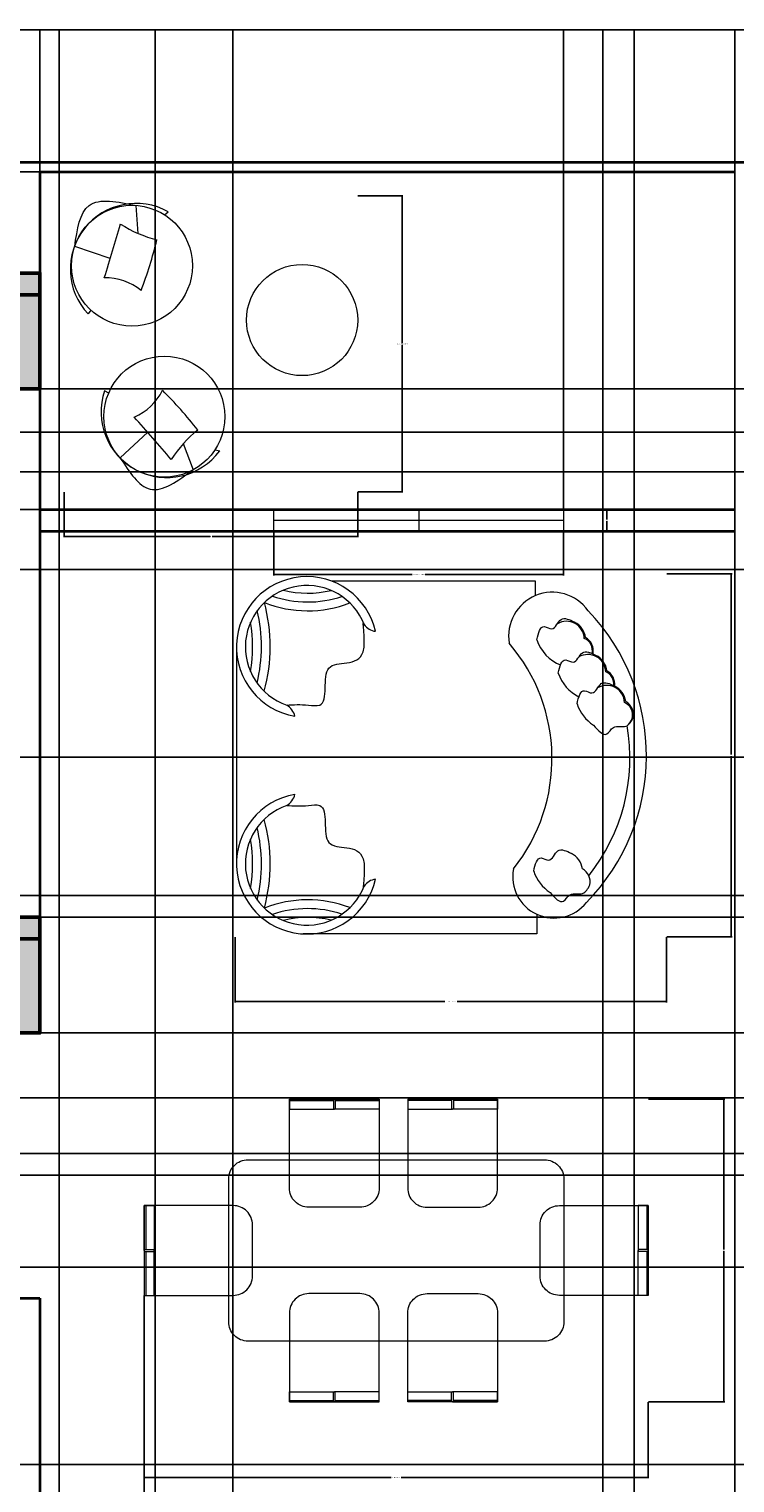
# Model space of a CAD drawing. Units: inches. Extents: x 393 to 993, y 153 to 660.
# Tile 4 of 6: x 645 to 791, y 359 to 660. Entities that reach past the tile are written whole.
import ezdxf

# ---------------------------------------------------------------- set-up
doc = ezdxf.new("R2010")
doc.units = ezdxf.units.IN
doc.header["$MEASUREMENT"] = 0
for name, color, linetype, lineweight in [('A-ANNO-DIMS', 2, 'Continuous', 18), ('A-COLS', 40, 'Continuous', 50), ('A-GLAZ', 4, 'Continuous', 20), ('A-WALL', 40, 'Continuous', 35), ('FURNITURE', 72, 'Continuous', 18)]:
    doc.layers.add(name, color=color, linetype=linetype, lineweight=lineweight)
doc.styles.get("Standard").update_dxf_attribs({"font": 'arial.ttf'})
doc.dimstyles.get("Standard").update_dxf_attribs({"dimtxt": 0.18, "dimasz": 0.18, "dimexe": 0.18, "dimexo": 0.0625, "dimgap": 0.09, "dimtad": 0, "dimtih": 1, "dimtoh": 1, "dimdec": 1, "dimzin": 0, "dimdsep": 46, "dimlunit": 3, "dimtxsty": 'Standard', "dimcen": 0.09, "dimadec": 0, "dimazin": 0, "dimtfac": 1, "dimtdec": 1, "dimtofl": 0, "dimtmove": 0, "dimatfit": 3, "dimfxl": 1, "dimtolj": 1, "dimtzin": 0, "dimarcsym": 0})

# ---------------------------------------------------------------- blocks, each defined once
blk = doc.blocks.new('YY')
for p, q in [((725.97, 560.91), (725.97, 558.66)), ((695.97, 558.66), (725.97, 558.66)), ((725.97, 558.66), (725.97, 556.41)), ((725.97, 558.66), (755.97, 558.66))]:
    blk.add_line(p, q)
blk.add_lwpolyline([(695.97, 556.41), (695.97, 560.91), (755.97, 560.91), (755.97, 556.41), (695.97, 556.41)])
blk = doc.blocks.new('SS')
for p, q in [((702.19, 481.41), (711.3, 481.41)), ((711.3, 481.71), (711.3, 479.62)), ((711.7, 481.71), (711.7, 479.62)), ((711.7, 481.41), (720.8, 481.41)), ((735.8, 481.41), (726.7, 481.41)), ((735.8, 481.71), (735.8, 479.62)), ((736.2, 481.71), (736.2, 479.62)), ((745.31, 481.41), (736.2, 481.41)), ((672.41, 459.62), (672.41, 450.52)), ((776.25, 459.62), (776.25, 450.52)), ((672.11, 450.52), (674.19, 450.52)), ((672.11, 450.12), (674.19, 450.12)), ((672.41, 450.12), (672.41, 441.01)), ((776.55, 450.52), (774.47, 450.52)), ((776.55, 450.12), (774.47, 450.12)), ((776.25, 450.12), (776.25, 441.01)), ((702.19, 419.23), (711.3, 419.23)), ((711.3, 418.93), (711.3, 421.02)), ((711.7, 418.93), (711.7, 421.02)), ((711.7, 419.23), (720.8, 419.23)), ((735.8, 419.23), (726.7, 419.23)), ((735.8, 418.93), (735.8, 421.02)), ((736.2, 418.93), (736.2, 421.02)), ((745.31, 419.23), (736.2, 419.23))]:
    blk.add_line(p, q)
for points in [[(702.19, 481.71), (720.8, 481.71), (720.8, 463.27, -0.414214), (716.8, 459.27), (706.19, 459.27, -0.414214), (702.19, 463.27)], [(745.31, 481.71), (726.7, 481.71), (726.7, 463.27, 0.414214), (730.7, 459.27), (741.31, 459.27, 0.414214), (745.31, 463.27)], [(693.61, 469.12), (755.05, 469.12, -0.414214), (759.05, 465.12), (759.05, 435.52, -0.414214), (755.05, 431.52), (693.61, 431.52, -0.414214), (689.61, 435.52), (689.61, 465.12, -0.414214)], [(672.11, 459.62), (672.11, 441.01), (690.54, 441.01, 0.414214), (694.54, 445.01), (694.54, 455.62, 0.414214), (690.54, 459.62)], [(776.55, 459.62), (776.55, 441.01), (758.12, 441.01, -0.414214), (754.12, 445.01), (754.12, 455.62, -0.414214), (758.12, 459.62)], [(702.19, 418.93), (720.8, 418.93), (720.8, 437.36, 0.414214), (716.8, 441.36), (706.19, 441.36, 0.414214), (702.19, 437.36)], [(745.31, 418.93), (726.7, 418.93), (726.7, 437.36, -0.414214), (730.7, 441.36), (741.31, 441.36, -0.414214), (745.31, 437.36)]]:
    blk.add_lwpolyline(points, format="xyb", close=True)
for points in [[(711.5, 481.71), (702.19, 481.71), (702.19, 479.62), (711.5, 479.62)], [(711.5, 481.71), (720.8, 481.71), (720.8, 479.62), (711.5, 479.62)], [(736, 481.71), (726.7, 481.71), (726.7, 479.62), (736, 479.62)], [(736, 481.71), (745.31, 481.71), (745.31, 479.62), (736, 479.62)], [(672.11, 450.32), (672.11, 459.62), (674.19, 459.62), (674.19, 450.32)], [(776.55, 450.32), (776.55, 459.62), (774.47, 459.62), (774.47, 450.32)], [(672.11, 450.32), (672.11, 441.01), (674.19, 441.01), (674.19, 450.32)], [(776.55, 450.32), (776.55, 441.01), (774.47, 441.01), (774.47, 450.32)], [(711.5, 418.93), (702.19, 418.93), (702.19, 421.02), (711.5, 421.02)], [(711.5, 418.93), (720.8, 418.93), (720.8, 421.02), (711.5, 421.02)], [(736, 418.93), (726.7, 418.93), (726.7, 421.02), (736, 421.02)], [(736, 418.93), (745.31, 418.93), (745.31, 421.02), (736, 421.02)]]:
    blk.add_lwpolyline(points)
blk = doc.blocks.new('CC')
for p, q in [((667.82, 618.13), (667.42, 623.92)), ((673.29, 621.98), (674.07, 622.6)), ((662.05, 612.95), (654.68, 615.45)), ((658.03, 602.24), (657.45, 601.43)), ((661.73, 585.02), (660.87, 585.52)), ((669.8, 576.91), (664.12, 571.6)), ((677.19, 574.56), (679.21, 569.12)), ((683.76, 573.3), (684.73, 573.06))]:
    blk.add_line(p, q)
for centre, radius in [((666.54, 611.43), 12.53), ((701.8, 600.17), 11.52), ((673.27, 580.15), 12.53)]:
    blk.add_circle(centre, radius)
for centre, radius, start, end in [((667.39, 610.73), 13.62, 60.6306, 223.0738), ((-908.47, 1091.34), 1641.76, 342.91261, 343.31902), ((677.83, 641.08), 25.04, 237.0171, 255.8371), ((587.69, 637.23), 86.46, 339.0342, 346.3342), ((660.99, 597.14), 11.8, 50.9057, 90.8219), ((673.76, 581.14), 13.62, 161.2133, 323.6564), ((662.33, 590.89), 11.8, 293.4651, 333.3813), ((612.01, 524.2), 86.46, 37.9528, 45.2528), ((-564.96, -505.1), 1641.76, 40.968, 41.3744), ((695.76, 557.76), 25.04, 128.4499, 147.2699)]:
    blk.add_arc(centre, radius, start, end)
for points in [[(654.68, 615.45), (655.2, 618.95), (656.28, 626.24), (663.61, 624.72), (667.42, 623.92)], [(664.12, 571.6), (666.03, 568.63), (670.01, 562.43), (676.06, 566.83), (679.21, 569.12)]]:
    blk.add_open_spline(points, degree=3, knots=[0, 0, 0, 0, 8.969281, 18.721099, 18.721099, 18.721099, 18.721099])
blk = doc.blocks.new('ll')
at = {"layer": 'FURNITURE'}
for p, q in [((750.18, 546.06), (707.9, 546.06)), ((750.18, 543.06), (750.18, 546.06)), ((688.21, 532.4), (688.21, 487.49)), ((750.42, 477.01), (750.42, 472.96)), ((750.42, 472.96), (702.01, 472.96))]:
    blk.add_line(p, q, dxfattribs=at)
for centre, radius, start, end in [((702.79, 532.4), 14.58, 12.8767, 260.2291), ((702.79, 532.4), 12.75, 21.3555, 250.8998), ((702.95, 564.16), 22.43, 250.9613, 288.4654), ((702.95, 564.16), 20.6, 255.8439, 283.5828), ((753.65, 534.69), 9.06, 35.3162, 189.6304), ((660.81, 532.52), 32.56, 346.4953, 13.1907), ((660.81, 532.52), 34.39, 344.3453, 15.3407), ((702.95, 564.16), 24.26, 248.2968, 291.1299), ((729.74, 509.85), 43.41, 315.5068, 43.8598), ((660.81, 532.52), 30.73, 350.2595, 9.4265), ((717.38, 538.95), 3.32, 214.9691, 263.4589), ((756.58, 534.03), 3.7, 2.2519, 120.5397), ((756.43, 533.85), 4.13, 7.2046, 63.8494), ((758.42, 536.54), 8.42, 198.3753, 248.7655), ((759.17, 531.63), 2.78, 348.3194, 66.5647), ((758.97, 531.6), 3.17, 349.5851, 60.6705), ((716.9, 509.26), 36.68, 321.4717, 40.6866), ((761.02, 527.14), 3.7, 2.2519, 120.5397), ((760.86, 526.95), 4.13, 7.2046, 63.8494), ((763.41, 524.7), 3.17, 352.5529, 60.6705), ((762.86, 529.64), 8.42, 198.3753, 243.944), ((764.92, 520.75), 3.7, 2.2519, 120.5397), ((763.61, 524.73), 2.78, 352.8755, 66.5647), ((763.61, 524.73), 2.78, 348.3194, 348.3993), ((764.76, 520.57), 4.13, 7.2046, 63.8494), ((696.54, 517.06), 3.9, 14.5272, 57.8422), ((766.76, 523.26), 8.42, 198.3753, 236.9846), ((767.51, 518.34), 2.78, 305.7015, 66.5647), ((767.31, 518.32), 3.17, 349.5851, 60.6705), ((730.58, 509.37), 39.14, 321.4898, 9.8869), ((702.79, 487.49), 14.58, 99.7709, 347.1233), ((696.54, 502.84), 3.9, 302.1578, 345.4728), ((702.79, 487.49), 12.75, 109.1002, 338.6445), ((660.81, 487.38), 32.56, 346.8093, 13.5047), ((660.81, 487.38), 34.39, 344.6593, 15.6547), ((660.81, 487.38), 30.73, 350.5735, 9.7405), ((755.78, 485.9), 4.13, 7.2046, 63.8494), ((754.02, 484.79), 8.58, 169.1466, 321.2907), ((757.78, 488.59), 8.42, 198.3753, 236.9846), ((758.33, 483.65), 3.17, 349.5851, 60.6705), ((717.38, 480.95), 3.32, 96.5411, 145.0309), ((702.95, 455.74), 24.26, 68.8701, 111.7032), ((702.95, 455.74), 22.43, 71.5346, 109.0387), ((702.95, 455.74), 20.6, 76.4172, 104.1561)]:
    blk.add_arc(centre, radius, start, end, dxfattribs=at)
for points, knots in [([(698.62, 520.36), (700.04, 520.44), (702.22, 520.56), (707.91, 519.62), (704.27, 531.4), (716.71, 526.93), (714.02, 538.83), (714.69, 536.96), (714.71, 536.92)], [0, 0, 0, 0, 4.487467, 6.830013, 14.741049, 22.564713, 28.22617, 28.364822, 28.364822, 28.364822, 28.364822]), ([(750.43, 533.89), (750.76, 535.31), (751.27, 537.45), (754.08, 535.39), (755.19, 539.08), (757.21, 538.07), (758.25, 537.56)], [0, 0, 0, 0, 3.161517, 4.748893, 7.471418, 10.321278, 10.321278, 10.321278, 10.321278]), ([(754.86, 526.99), (755.2, 528.41), (755.71, 530.55), (758.51, 528.49), (759.63, 532.18), (761.65, 531.17), (762.68, 530.66)], [0, 0, 0, 0, 3.161517, 4.748893, 7.471418, 10.321278, 10.321278, 10.321278, 10.321278]), ([(758.77, 520.6), (759.1, 522.03), (759.61, 524.16), (762.42, 522.1), (763.53, 525.79), (765.55, 524.79), (766.59, 524.28)], [0, 0, 0, 0, 3.161517, 4.748893, 7.471418, 10.321278, 10.321278, 10.321278, 10.321278]), ([(762.17, 516.19), (763.19, 515.06), (764.77, 513.29), (766.27, 516.46), (769.11, 515.35), (770.01, 516.98), (770.43, 517.75)], [0, 0, 0, 0, 3.335346, 5.221215, 7.830033, 10.164656, 10.164656, 10.164656, 10.164656]), ([(698.62, 499.54), (700.04, 499.46), (702.22, 499.34), (707.91, 500.28), (704.27, 488.5), (716.71, 492.97), (714.02, 481.06), (714.69, 482.94), (714.71, 482.98)], [0, 0, 0, 0, 4.487467, 6.830013, 14.741049, 22.564713, 28.22617, 28.364822, 28.364822, 28.364822, 28.364822]), ([(749.79, 485.93), (750.12, 487.36), (750.63, 489.49), (753.43, 487.43), (754.55, 491.12), (756.57, 490.12), (757.61, 489.61)], [0, 0, 0, 0, 3.161517, 4.748893, 7.471418, 10.321278, 10.321278, 10.321278, 10.321278]), ([(753.19, 481.52), (754.21, 480.39), (755.79, 478.62), (757.28, 481.79), (760.13, 480.68), (761.03, 482.31), (761.45, 483.08)], [0, 0, 0, 0, 3.335346, 5.221215, 7.830033, 10.164656, 10.164656, 10.164656, 10.164656])]:
    blk.add_open_spline(points, degree=3, knots=knots, dxfattribs=at)
blk = doc.blocks.new('COL-9X24-RH')
h = blk.add_hatch(color=256)
h.dxf.hatch_style = 1
h.paths.add_polyline_path([(4.5, 19.5), (4.5, 24), (0, 24), (0, 0), (9, 0), (9, 19.5)])
h = blk.add_hatch(color=256)
h.dxf.hatch_style = 1
h.paths.add_polyline_path([(4.5, 19.5), (9, 19.5), (9, 24), (4.5, 24)])
for p, q in [((4.5, 24), (4.5, 19.5)), ((4.5, 24), (9, 24)), ((9, 24), (9, 19.5)), ((4.5, 19.5), (9, 19.5))]:
    blk.add_line(p, q)
blk.add_lwpolyline([(0, 24), (9, 24), (9, 0), (0, 0), (0, 24)])
blk = doc.blocks.new('*D28')
at = {"layer": 'A-ANNO-DIMS', "color": 0, "lineweight": -2, "transparency": 16777216}
for p, q in [((695.97, 556.34), (695.97, 547.23)), ((755.97, 556.34), (755.97, 547.23)), ((696.15, 547.41), (724.63, 547.41)), ((755.79, 547.41), (727.31, 547.41))]:
    blk.add_line(p, q, dxfattribs=at)
at = {"layer": 'A-ANNO-DIMS', "color": 0, "transparency": 16777216}
for points in [[(696.15, 547.44), (696.15, 547.38), (695.97, 547.41)], [(755.79, 547.44), (755.79, 547.38), (755.97, 547.41)]]:
    blk.add_solid(points, dxfattribs=at)
at = {"layer": 'Defpoints', "color": 0, "transparency": 16777216}
for p in [(695.97, 556.41), (755.97, 556.41), (755.97, 547.41)]:
    blk.add_point(p, dxfattribs=at)
at = {"layer": 'A-ANNO-DIMS', "color": 0, "transparency": 16777216, "insert": (725.97, 547.41), "char_height": 0.18, "attachment_point": 5}
blk.add_mtext('\\A1;BALCONY SLIDER 60', dxfattribs=at)
blk = doc.blocks.new('*D29')
at = {"layer": 'A-ANNO-DIMS', "color": 0, "lineweight": -2, "transparency": 16777216}
for p, q in [((756.03, 560.91), (765.15, 560.91)), ((764.97, 560.73), (764.97, 558.84)), ((764.97, 556.59), (764.97, 558.48)), ((756.03, 556.41), (765.15, 556.41))]:
    blk.add_line(p, q, dxfattribs=at)
at = {"layer": 'A-ANNO-DIMS', "color": 0, "transparency": 16777216}
for points in [[(764.94, 560.73), (765, 560.73), (764.97, 560.91)], [(764.94, 556.59), (765, 556.59), (764.97, 556.41)]]:
    blk.add_solid(points, dxfattribs=at)
at = {"layer": 'Defpoints', "color": 0, "transparency": 16777216}
for p in [(755.97, 560.91), (764.97, 560.91), (755.97, 556.41)]:
    blk.add_point(p, dxfattribs=at)
at = {"layer": 'A-ANNO-DIMS', "color": 0, "transparency": 16777216, "insert": (764.97, 558.66), "char_height": 0.18, "attachment_point": 5}
blk.add_mtext('\\A1;5', dxfattribs=at)
blk = doc.blocks.new('*D36')
at = {"layer": 'A-ANNO-DIMS', "color": 0, "lineweight": -2, "transparency": 16777216}
for p, q in [((669.09, 375.86), (669.09, 360.08)), ((773.53, 375.86), (773.53, 360.08)), ((669.27, 360.26), (720.27, 360.26)), ((773.35, 360.26), (722.35, 360.26))]:
    blk.add_line(p, q, dxfattribs=at)
at = {"layer": 'A-ANNO-DIMS', "color": 0, "transparency": 16777216}
for points in [[(669.27, 360.29), (669.27, 360.23), (669.09, 360.26)], [(773.35, 360.29), (773.35, 360.23), (773.53, 360.26)]]:
    blk.add_solid(points, dxfattribs=at)
at = {"layer": 'Defpoints', "color": 0, "transparency": 16777216}
for p in [(669.09, 375.92), (773.53, 375.92), (773.53, 360.26)]:
    blk.add_point(p, dxfattribs=at)
at = {"layer": 'A-ANNO-DIMS', "color": 0, "transparency": 16777216, "insert": (721.31, 360.26), "char_height": 0.18, "attachment_point": 5}
blk.add_mtext('\\A1;DINING SET 104', dxfattribs=at)
blk = doc.blocks.new('*D37')
at = {"layer": 'A-ANNO-DIMS', "color": 0, "lineweight": -2, "transparency": 16777216}
for p, q in [((773.6, 438.7), (789.38, 438.7)), ((789.2, 438.52), (789.2, 407.49)), ((789.2, 376.1), (789.2, 407.13)), ((773.6, 375.92), (789.38, 375.92))]:
    blk.add_line(p, q, dxfattribs=at)
at = {"layer": 'A-ANNO-DIMS', "color": 0, "transparency": 16777216}
for points in [[(789.17, 438.52), (789.23, 438.52), (789.2, 438.7)], [(789.17, 376.1), (789.23, 376.1), (789.2, 375.92)]]:
    blk.add_solid(points, dxfattribs=at)
at = {"layer": 'Defpoints', "color": 0, "transparency": 16777216}
for p in [(773.53, 438.7), (789.2, 438.7), (773.53, 375.92)]:
    blk.add_point(p, dxfattribs=at)
at = {"layer": 'A-ANNO-DIMS', "color": 0, "transparency": 16777216, "insert": (789.2, 407.31), "char_height": 0.18, "attachment_point": 5}
blk.add_mtext('\\A1;63', dxfattribs=at)
blk = doc.blocks.new('*D38')
at = {"layer": 'A-ANNO-DIMS', "color": 0, "lineweight": -2, "transparency": 16777216}
for p, q in [((713.38, 625.89), (722.7, 625.89)), ((722.52, 625.71), (722.52, 595.4)), ((722.52, 564.72), (722.52, 595.03)), ((713.38, 564.54), (722.7, 564.54))]:
    blk.add_line(p, q, dxfattribs=at)
at = {"layer": 'A-ANNO-DIMS', "color": 0, "transparency": 16777216}
for points in [[(722.49, 625.71), (722.55, 625.71), (722.52, 625.89)], [(722.49, 564.72), (722.55, 564.72), (722.52, 564.54)]]:
    blk.add_solid(points, dxfattribs=at)
at = {"layer": 'Defpoints', "color": 0, "transparency": 16777216}
for p in [(713.32, 625.89), (722.52, 625.89), (713.32, 564.54)]:
    blk.add_point(p, dxfattribs=at)
at = {"layer": 'A-ANNO-DIMS', "color": 0, "transparency": 16777216, "insert": (722.52, 595.22), "char_height": 0.18, "attachment_point": 5}
blk.add_mtext('\\A1;BALCONY SEATING 61', dxfattribs=at)
blk = doc.blocks.new('*D39')
at = {"layer": 'A-ANNO-DIMS', "color": 0, "lineweight": -2, "transparency": 16777216}
for p, q in [((652.53, 564.48), (652.53, 555.15)), ((713.32, 564.48), (713.32, 555.15)), ((652.71, 555.33), (682.72, 555.33)), ((713.14, 555.33), (683.13, 555.33))]:
    blk.add_line(p, q, dxfattribs=at)
at = {"layer": 'A-ANNO-DIMS', "color": 0, "transparency": 16777216}
for points in [[(652.71, 555.36), (652.71, 555.3), (652.53, 555.33)], [(713.14, 555.36), (713.14, 555.3), (713.32, 555.33)]]:
    blk.add_solid(points, dxfattribs=at)
at = {"layer": 'Defpoints', "color": 0, "transparency": 16777216}
for p in [(652.53, 564.54), (713.32, 564.54), (713.32, 555.33)]:
    blk.add_point(p, dxfattribs=at)
at = {"layer": 'A-ANNO-DIMS', "color": 0, "transparency": 16777216, "insert": (682.92, 555.33), "char_height": 0.18, "attachment_point": 5}
blk.add_mtext('\\A1;61', dxfattribs=at)
blk = doc.blocks.new('*D40')
at = {"layer": 'A-ANNO-DIMS', "color": 0, "lineweight": -2, "transparency": 16777216}
for p, q in [((687.93, 472.24), (687.93, 458.71)), ((777.32, 472.24), (777.32, 458.71)), ((688.11, 458.89), (731.35, 458.89)), ((777.14, 458.89), (733.9, 458.89))]:
    blk.add_line(p, q, dxfattribs=at)
at = {"layer": 'A-ANNO-DIMS', "color": 0, "transparency": 16777216}
for points in [[(688.11, 458.92), (688.11, 458.86), (687.93, 458.89)], [(777.14, 458.92), (777.14, 458.86), (777.32, 458.89)]]:
    blk.add_solid(points, dxfattribs=at)
at = {"layer": 'Defpoints', "color": 0, "transparency": 16777216}
for p in [(687.93, 472.3), (777.32, 472.3), (777.32, 458.89)]:
    blk.add_point(p, dxfattribs=at)
at = {"layer": 'A-ANNO-DIMS', "color": 0, "transparency": 16777216, "insert": (732.63, 458.89), "char_height": 0.18, "attachment_point": 5}
blk.add_mtext('\\A1;LOUNGE GROUP 89', dxfattribs=at)
blk = doc.blocks.new('*D41')
at = {"layer": 'A-ANNO-DIMS', "color": 0, "lineweight": -2, "transparency": 16777216}
for p, q in [((777.38, 547.6), (790.9, 547.6)), ((790.72, 547.42), (790.72, 510.13)), ((790.72, 472.48), (790.72, 509.77)), ((777.38, 472.3), (790.9, 472.3))]:
    blk.add_line(p, q, dxfattribs=at)
at = {"layer": 'A-ANNO-DIMS', "color": 0, "transparency": 16777216}
for points in [[(790.69, 547.42), (790.75, 547.42), (790.72, 547.6)], [(790.69, 472.48), (790.75, 472.48), (790.72, 472.3)]]:
    blk.add_solid(points, dxfattribs=at)
at = {"layer": 'Defpoints', "color": 0, "transparency": 16777216}
for p in [(777.32, 547.6), (790.72, 547.6), (777.32, 472.3)]:
    blk.add_point(p, dxfattribs=at)
at = {"layer": 'A-ANNO-DIMS', "color": 0, "transparency": 16777216, "insert": (790.72, 509.95), "char_height": 0.18, "attachment_point": 5}
blk.add_mtext('\\A1;75', dxfattribs=at)
blk = doc.blocks.new('*D48')
at = {"layer": 'A-ANNO-DIMS', "color": 0, "lineweight": -2, "transparency": 16777216}
for p, q in [((642.98, 632.97), (642.98, 660.49)), ((643.16, 660.31), (719.2, 660.31)), ((795.8, 660.31), (719.76, 660.31)), ((795.98, 632.97), (795.98, 660.49))]:
    blk.add_line(p, q, dxfattribs=at)
at = {"layer": 'A-ANNO-DIMS', "color": 0, "transparency": 16777216}
for points in [[(643.16, 660.34), (643.16, 660.28), (642.98, 660.31)], [(795.8, 660.34), (795.8, 660.28), (795.98, 660.31)]]:
    blk.add_solid(points, dxfattribs=at)
at = {"layer": 'Defpoints', "color": 0, "transparency": 16777216}
for p in [(795.98, 660.31), (642.98, 632.91), (795.98, 632.91)]:
    blk.add_point(p, dxfattribs=at)
at = {"layer": 'A-ANNO-DIMS', "color": 0, "transparency": 16777216, "insert": (719.48, 660.31), "char_height": 0.18, "attachment_point": 5}
blk.add_mtext('\\A1;153', dxfattribs=at)
blk = doc.blocks.new('*D55')
at = {"layer": 'A-ANNO-DIMS', "color": 0, "lineweight": -2, "transparency": 16777216}
for p, q in [((791.42, 630.91), (393.4, 630.91)), ((393.58, 630.73), (393.58, 596.09)), ((393.58, 561.09), (393.58, 595.72)), ((791.42, 560.91), (393.4, 560.91))]:
    blk.add_line(p, q, dxfattribs=at)
at = {"layer": 'A-ANNO-DIMS', "color": 0, "transparency": 16777216}
for points in [[(393.55, 630.73), (393.61, 630.73), (393.58, 630.91)], [(393.55, 561.09), (393.61, 561.09), (393.58, 560.91)]]:
    blk.add_solid(points, dxfattribs=at)
at = {"layer": 'Defpoints', "color": 0, "transparency": 16777216}
for p in [(791.48, 630.91), (393.58, 560.91), (791.48, 560.91)]:
    blk.add_point(p, dxfattribs=at)
at = {"layer": 'A-ANNO-DIMS', "color": 0, "transparency": 16777216, "insert": (393.58, 595.91), "char_height": 0.18, "attachment_point": 5}
blk.add_mtext('\\A1;70', dxfattribs=at)
blk = doc.blocks.new('*D59')
at = {"layer": 'A-ANNO-DIMS', "color": 0, "lineweight": -2, "transparency": 16777216}
for p, q in [((651.48, 185.47), (651.48, 660.49)), ((651.66, 660.31), (669.26, 660.31)), ((687.3, 660.31), (669.7, 660.31)), ((687.48, 185.47), (687.48, 660.49))]:
    blk.add_line(p, q, dxfattribs=at)
at = {"layer": 'A-ANNO-DIMS', "color": 0, "transparency": 16777216}
for points in [[(651.66, 660.34), (651.66, 660.28), (651.48, 660.31)], [(687.3, 660.34), (687.3, 660.28), (687.48, 660.31)]]:
    blk.add_solid(points, dxfattribs=at)
at = {"layer": 'Defpoints', "color": 0, "transparency": 16777216}
for p in [(687.48, 660.31), (651.48, 185.41), (687.48, 185.41)]:
    blk.add_point(p, dxfattribs=at)
at = {"layer": 'A-ANNO-DIMS', "color": 0, "transparency": 16777216, "insert": (669.48, 660.31), "char_height": 0.18, "attachment_point": 5}
blk.add_mtext('\\A1;36', dxfattribs=at)
blk = doc.blocks.new('*D62')
at = {"layer": 'A-ANNO-DIMS', "color": 0, "lineweight": -2, "transparency": 16777216}
for p, q in [((848.42, 422.91), (393.4, 422.91)), ((393.58, 422.73), (393.58, 393.09)), ((393.58, 363.09), (393.58, 392.72)), ((848.42, 362.91), (393.4, 362.91))]:
    blk.add_line(p, q, dxfattribs=at)
at = {"layer": 'A-ANNO-DIMS', "color": 0, "transparency": 16777216}
for points in [[(393.55, 422.73), (393.61, 422.73), (393.58, 422.91)], [(393.55, 363.09), (393.61, 363.09), (393.58, 362.91)]]:
    blk.add_solid(points, dxfattribs=at)
at = {"layer": 'Defpoints', "color": 0, "transparency": 16777216}
for p in [(393.58, 422.91), (848.48, 422.91), (848.48, 362.91)]:
    blk.add_point(p, dxfattribs=at)
at = {"layer": 'A-ANNO-DIMS', "color": 0, "transparency": 16777216, "insert": (393.58, 392.91), "char_height": 0.18, "attachment_point": 5}
blk.add_mtext('\\A1;60', dxfattribs=at)
blk = doc.blocks.new('*D63')
at = {"layer": 'A-ANNO-DIMS', "color": 0, "lineweight": -2, "transparency": 16777216}
for p, q in [((960.92, 476.41), (393.4, 476.41)), ((393.58, 476.23), (393.58, 452.09)), ((393.58, 427.59), (393.58, 451.72)), ((960.92, 427.41), (393.4, 427.41))]:
    blk.add_line(p, q, dxfattribs=at)
at = {"layer": 'A-ANNO-DIMS', "color": 0, "transparency": 16777216}
for points in [[(393.55, 476.23), (393.61, 476.23), (393.58, 476.41)], [(393.55, 427.59), (393.61, 427.59), (393.58, 427.41)]]:
    blk.add_solid(points, dxfattribs=at)
at = {"layer": 'Defpoints', "color": 0, "transparency": 16777216}
for p in [(393.58, 476.41), (960.98, 476.41), (960.98, 427.41)]:
    blk.add_point(p, dxfattribs=at)
at = {"layer": 'A-ANNO-DIMS', "color": 0, "transparency": 16777216, "insert": (393.58, 451.91), "char_height": 0.18, "attachment_point": 5}
blk.add_mtext('\\A1;49', dxfattribs=at)
blk = doc.blocks.new('*D64')
at = {"layer": 'A-ANNO-DIMS', "color": 0, "lineweight": -2, "transparency": 16777216}
for p, q in [((932.42, 576.91), (393.4, 576.91)), ((393.58, 576.73), (393.58, 529.09)), ((393.58, 481.09), (393.58, 528.72)), ((932.42, 480.91), (393.4, 480.91))]:
    blk.add_line(p, q, dxfattribs=at)
at = {"layer": 'A-ANNO-DIMS', "color": 0, "transparency": 16777216}
for points in [[(393.55, 576.73), (393.61, 576.73), (393.58, 576.91)], [(393.55, 481.09), (393.61, 481.09), (393.58, 480.91)]]:
    blk.add_solid(points, dxfattribs=at)
at = {"layer": 'Defpoints', "color": 0, "transparency": 16777216}
for p in [(393.58, 576.91), (932.48, 576.91), (932.48, 480.91)]:
    blk.add_point(p, dxfattribs=at)
at = {"layer": 'A-ANNO-DIMS', "color": 0, "transparency": 16777216, "insert": (393.58, 528.91), "char_height": 0.18, "attachment_point": 5}
blk.add_mtext('\\A1;96', dxfattribs=at)
blk = doc.blocks.new('*D67')
at = {"layer": 'A-ANNO-DIMS', "color": 0, "lineweight": -2, "transparency": 16777216}
for p, q in [((647.48, 452.47), (647.48, 660.49)), ((647.66, 660.31), (719.2, 660.31)), ((791.3, 660.31), (719.76, 660.31)), ((791.48, 427.47), (791.48, 660.49))]:
    blk.add_line(p, q, dxfattribs=at)
at = {"layer": 'A-ANNO-DIMS', "color": 0, "transparency": 16777216}
for points in [[(647.66, 660.34), (647.66, 660.28), (647.48, 660.31)], [(791.3, 660.34), (791.3, 660.28), (791.48, 660.31)]]:
    blk.add_solid(points, dxfattribs=at)
at = {"layer": 'Defpoints', "color": 0, "transparency": 16777216}
for p in [(791.48, 660.31), (647.48, 452.41), (791.48, 427.41)]:
    blk.add_point(p, dxfattribs=at)
at = {"layer": 'A-ANNO-DIMS', "color": 0, "transparency": 16777216, "insert": (719.48, 660.31), "char_height": 0.18, "attachment_point": 5}
blk.add_mtext('\\A1;144', dxfattribs=at)
blk = doc.blocks.new('*D68')
at = {"layer": 'A-ANNO-DIMS', "color": 0, "lineweight": -2, "transparency": 16777216}
for p, q in [((671.33, 314.02), (671.33, 660.49)), ((671.51, 660.31), (720.57, 660.31)), ((770.41, 660.31), (721.36, 660.31)), ((770.59, 314.02), (770.59, 660.49))]:
    blk.add_line(p, q, dxfattribs=at)
at = {"layer": 'A-ANNO-DIMS', "color": 0, "transparency": 16777216}
for points in [[(671.51, 660.34), (671.51, 660.28), (671.33, 660.31)], [(770.41, 660.34), (770.41, 660.28), (770.59, 660.31)]]:
    blk.add_solid(points, dxfattribs=at)
at = {"layer": 'Defpoints', "color": 0, "transparency": 16777216}
for p in [(770.59, 660.31), (671.33, 313.96), (770.59, 313.96)]:
    blk.add_point(p, dxfattribs=at)
at = {"layer": 'A-ANNO-DIMS', "color": 0, "transparency": 16777216, "insert": (720.96, 660.31), "char_height": 0.18, "attachment_point": 5}
blk.add_mtext('\\A1;99.26', dxfattribs=at)
blk = doc.blocks.new('*D72')
at = {"layer": 'A-ANNO-DIMS', "color": 0, "lineweight": -2, "transparency": 16777216}
for p, q in [((481.04, 452.41), (993.06, 452.41)), ((992.88, 452.23), (992.88, 445.86)), ((992.88, 439.14), (992.88, 445.5)), ((481.04, 438.96), (993.06, 438.96))]:
    blk.add_line(p, q, dxfattribs=at)
at = {"layer": 'A-ANNO-DIMS', "color": 0, "transparency": 16777216}
for points in [[(992.85, 452.23), (992.91, 452.23), (992.88, 452.41)], [(992.85, 439.14), (992.91, 439.14), (992.88, 438.96)]]:
    blk.add_solid(points, dxfattribs=at)
at = {"layer": 'Defpoints', "color": 0, "transparency": 16777216}
for p in [(480.98, 452.41), (992.88, 452.41), (480.98, 438.96)]:
    blk.add_point(p, dxfattribs=at)
at = {"layer": 'A-ANNO-DIMS', "color": 0, "transparency": 16777216, "insert": (992.88, 445.68), "char_height": 0.18, "attachment_point": 5}
blk.add_mtext('\\A1;13.45', dxfattribs=at)
blk = doc.blocks.new('*D73')
at = {"layer": 'A-ANNO-DIMS', "color": 0, "lineweight": -2, "transparency": 16777216}
for p, q in [((956.42, 422.91), (393.4, 422.91)), ((393.58, 422.73), (393.58, 413.55)), ((393.58, 404.01), (393.58, 413.19)), ((956.42, 403.83), (393.4, 403.83))]:
    blk.add_line(p, q, dxfattribs=at)
at = {"layer": 'A-ANNO-DIMS', "color": 0, "transparency": 16777216}
for points in [[(393.55, 422.73), (393.61, 422.73), (393.58, 422.91)], [(393.55, 404.01), (393.61, 404.01), (393.58, 403.83)]]:
    blk.add_solid(points, dxfattribs=at)
at = {"layer": 'Defpoints', "color": 0, "transparency": 16777216}
for p in [(393.58, 422.91), (956.48, 422.91), (956.48, 403.83)]:
    blk.add_point(p, dxfattribs=at)
at = {"layer": 'A-ANNO-DIMS', "color": 0, "transparency": 16777216, "insert": (393.58, 413.37), "char_height": 0.18, "attachment_point": 5}
blk.add_mtext('\\A1;19.08', dxfattribs=at)
blk = doc.blocks.new('*D74')
at = {"layer": 'A-ANNO-DIMS', "color": 0, "lineweight": -2, "transparency": 16777216}
for p, q in [((956.42, 585.91), (393.4, 585.91)), ((393.58, 585.73), (393.58, 577.48)), ((393.58, 568.88), (393.58, 577.12)), ((956.42, 568.7), (393.4, 568.7))]:
    blk.add_line(p, q, dxfattribs=at)
at = {"layer": 'A-ANNO-DIMS', "color": 0, "transparency": 16777216}
for points in [[(393.55, 585.73), (393.61, 585.73), (393.58, 585.91)], [(393.55, 568.88), (393.61, 568.88), (393.58, 568.7)]]:
    blk.add_solid(points, dxfattribs=at)
at = {"layer": 'Defpoints', "color": 0, "transparency": 16777216}
for p in [(393.58, 585.91), (956.48, 585.91), (956.48, 568.7)]:
    blk.add_point(p, dxfattribs=at)
at = {"layer": 'A-ANNO-DIMS', "color": 0, "transparency": 16777216, "insert": (393.58, 577.3), "char_height": 0.18, "attachment_point": 5}
blk.add_mtext('\\A1;17.21', dxfattribs=at)
blk = doc.blocks.new('*D75')
at = {"layer": 'A-ANNO-DIMS', "color": 0, "lineweight": -2, "transparency": 16777216}
for p, q in [((764.1, 185.47), (764.1, 660.49)), ((764.28, 660.31), (777.39, 660.31)), ((791.3, 660.31), (778.19, 660.31)), ((791.48, 185.47), (791.48, 660.49))]:
    blk.add_line(p, q, dxfattribs=at)
at = {"layer": 'A-ANNO-DIMS', "color": 0, "transparency": 16777216}
for points in [[(764.28, 660.34), (764.28, 660.28), (764.1, 660.31)], [(791.3, 660.34), (791.3, 660.28), (791.48, 660.31)]]:
    blk.add_solid(points, dxfattribs=at)
at = {"layer": 'Defpoints', "color": 0, "transparency": 16777216}
for p in [(791.48, 660.31), (764.1, 185.41), (791.48, 185.41)]:
    blk.add_point(p, dxfattribs=at)
at = {"layer": 'A-ANNO-DIMS', "color": 0, "transparency": 16777216, "insert": (777.79, 660.31), "char_height": 0.18, "attachment_point": 5}
blk.add_mtext('\\A1;27.38', dxfattribs=at)
blk = doc.blocks.new('*D76')
at = {"layer": 'A-ANNO-DIMS', "color": 0, "lineweight": -2, "transparency": 16777216}
for p, q in [((755.97, 560.97), (755.97, 660.49)), ((756.15, 660.31), (773.35, 660.31)), ((791.3, 660.31), (774.1, 660.31)), ((791.48, 560.97), (791.48, 660.49))]:
    blk.add_line(p, q, dxfattribs=at)
at = {"layer": 'A-ANNO-DIMS', "color": 0, "transparency": 16777216}
for points in [[(756.15, 660.34), (756.15, 660.28), (755.97, 660.31)], [(791.3, 660.34), (791.3, 660.28), (791.48, 660.31)]]:
    blk.add_solid(points, dxfattribs=at)
at = {"layer": 'Defpoints', "color": 0, "transparency": 16777216}
for p in [(791.48, 660.31), (755.97, 560.91), (791.48, 560.91)]:
    blk.add_point(p, dxfattribs=at)
at = {"layer": 'A-ANNO-DIMS', "color": 0, "transparency": 16777216, "insert": (773.72, 660.31), "char_height": 0.18, "attachment_point": 5}
blk.add_mtext('\\A1;35.51', dxfattribs=at)
blk = doc.blocks.new('*D80')
at = {"layer": 'A-ANNO-DIMS', "color": 0, "lineweight": -2, "transparency": 16777216}
for p, q in [((879.42, 480.91), (393.4, 480.91)), ((393.58, 480.73), (393.58, 478.84)), ((879.42, 476.41), (393.4, 476.41)), ((393.58, 476.59), (393.58, 478.48))]:
    blk.add_line(p, q, dxfattribs=at)
at = {"layer": 'A-ANNO-DIMS', "color": 0, "transparency": 16777216}
for points in [[(393.55, 480.73), (393.61, 480.73), (393.58, 480.91)], [(393.55, 476.59), (393.61, 476.59), (393.58, 476.41)]]:
    blk.add_solid(points, dxfattribs=at)
at = {"layer": 'Defpoints', "color": 0, "transparency": 16777216}
for p in [(393.58, 480.91), (879.48, 480.91), (879.48, 476.41)]:
    blk.add_point(p, dxfattribs=at)
at = {"layer": 'A-ANNO-DIMS', "color": 0, "transparency": 16777216, "insert": (393.58, 478.66), "char_height": 0.18, "attachment_point": 5}
blk.add_mtext('\\A1;4.5', dxfattribs=at)
blk = doc.blocks.new('*D81')
at = {"layer": 'A-ANNO-DIMS', "color": 0, "lineweight": -2, "transparency": 16777216}
for p, q in [((669.09, 397.94), (669.09, 153.33)), ((647.48, 397.34), (647.48, 153.33)), ((647.66, 153.51), (657.91, 153.51)), ((668.91, 153.51), (658.66, 153.51))]:
    blk.add_line(p, q, dxfattribs=at)
at = {"layer": 'A-ANNO-DIMS', "color": 0, "transparency": 16777216}
for points in [[(647.66, 153.54), (647.66, 153.48), (647.48, 153.51)], [(668.91, 153.54), (668.91, 153.48), (669.09, 153.51)]]:
    blk.add_solid(points, dxfattribs=at)
at = {"layer": 'Defpoints', "color": 0, "transparency": 16777216}
for p in [(669.09, 398.01), (647.48, 397.41), (669.09, 153.51)]:
    blk.add_point(p, dxfattribs=at)
at = {"layer": 'A-ANNO-DIMS', "color": 0, "transparency": 16777216, "insert": (658.29, 153.51), "char_height": 0.18, "attachment_point": 5}
blk.add_mtext('\\A1;21.61', dxfattribs=at)
blk = doc.blocks.new('*D84')
at = {"layer": 'A-ANNO-DIMS', "color": 0, "lineweight": -2, "transparency": 16777216}
for p, q in [((956.42, 548.43), (393.4, 548.43)), ((393.58, 548.25), (393.58, 529.18)), ((393.58, 509.74), (393.58, 528.81)), ((956.42, 509.56), (393.4, 509.56))]:
    blk.add_line(p, q, dxfattribs=at)
at = {"layer": 'A-ANNO-DIMS', "color": 0, "transparency": 16777216}
for points in [[(393.55, 548.25), (393.61, 548.25), (393.58, 548.43)], [(393.55, 509.74), (393.61, 509.74), (393.58, 509.56)]]:
    blk.add_solid(points, dxfattribs=at)
at = {"layer": 'Defpoints', "color": 0, "transparency": 16777216}
for p in [(393.58, 548.43), (956.48, 548.43), (956.48, 509.56)]:
    blk.add_point(p, dxfattribs=at)
at = {"layer": 'A-ANNO-DIMS', "color": 0, "transparency": 16777216, "insert": (393.58, 529), "char_height": 0.18, "attachment_point": 5}
blk.add_mtext('\\A1;38.87', dxfattribs=at)

msp = doc.modelspace()

# ---------------------------------------------------------------- linework, layer by layer
at = {"layer": 'A-WALL'}
for p, q in [((642.9798, 632.9066), (795.9798, 632.9066)), ((647.4798, 630.9066), (647.4798, 452.4066)), ((647.4798, 630.9066), (791.4798, 630.9066)), ((647.4798, 560.9066), (791.4798, 560.9066)), ((647.4798, 556.4066), (791.4798, 556.4066)), ((642.9798, 397.4066), (647.4798, 397.4066)), ((647.4798, 397.4066), (647.4798, 314.9066))]:
    msp.add_line(p, q, dxfattribs=at)

# ---------------------------------------------------------------- block references
at = {"layer": 'A-COLS'}
for p in [(638.48, 585.907), (638.48, 452.407)]:
    msp.add_blockref('COL-9X24-RH', p, dxfattribs=at)
at = {"layer": 'A-GLAZ'}
msp.add_blockref('YY', (0, 0), dxfattribs=at)
at = {"layer": 'FURNITURE'}
for name, p in [('CC', (0, 0)), ('ll', (0, 0)), ('SS', (-3.0181, -43.0062))]:
    msp.add_blockref(name, p, dxfattribs=at)

# ---------------------------------------------------------------- dimensions: what is measured, and where the dimension line sits
at = {"layer": 'A-ANNO-DIMS'}
for base, p1, p2, override, picture, middle in [((795.9798, 660.3066), (642.9798, 632.9066), (795.9798, 632.9066), {"dimdec": 0, "dimlfac": 1, "dimrnd": 0, "dimzin": 0, "dimdsep": 46, "dimlunit": 2}, '*D48', (719.4798, 660.3066)), ((791.4798, 660.3066), (647.4798, 452.4066), (791.4798, 427.4066), {"dimdec": 0, "dimlfac": 1, "dimrnd": 0, "dimzin": 0, "dimdsep": 46, "dimlunit": 2}, '*D67', (719.4798, 660.3066)), ((687.4798, 660.3066), (651.4798, 185.4066), (687.4798, 185.4066), {"dimdec": 0, "dimlfac": 1, "dimrnd": 0, "dimzin": 0, "dimdsep": 46, "dimlunit": 2}, '*D59', (669.4798, 660.3066)), ((770.5908, 660.3066), (671.3346, 313.958), (770.5908, 313.958), {"dimdec": 2, "dimlfac": 1, "dimrnd": 0, "dimzin": 0, "dimdsep": 46, "dimlunit": 2}, '*D68', (720.9627, 660.3066)), ((791.4798, 660.3066), (755.9701, 560.9066), (791.4798, 560.9066), {"dimdec": 2, "dimlfac": 1, "dimrnd": 0, "dimzin": 0, "dimdsep": 46, "dimlunit": 2}, '*D76', (773.7249, 660.3066)), ((791.4798, 660.3066), (764.1009, 185.4066), (791.4798, 185.4066), {"dimdec": 2, "dimlfac": 1, "dimrnd": 0, "dimzin": 0, "dimdsep": 46, "dimlunit": 2}, '*D75', (777.7904, 660.3066)), ((713.3168, 555.3341), (652.5326, 564.5376), (713.3168, 564.5376), {"dimdec": 0, "dimlfac": 1, "dimrnd": 0, "dimzin": 0, "dimdsep": 46, "dimlunit": 2}, '*D39', (682.9247, 555.3341)), ((669.0909, 153.5066), (647.4798, 397.4066), (669.0909, 398.0071), {"dimdec": 2, "dimlfac": 1, "dimrnd": 0, "dimzin": 0, "dimdsep": 46, "dimlunit": 2}, '*D81', (658.2853, 153.5066))]:
    dim = msp.add_linear_dim(base=base, p1=p1, p2=p2, dimstyle='Standard', override=override, dxfattribs=at)
    dim.commit()
    dim.dimension.update_dxf_attribs({"geometry": picture, "text_midpoint": middle})
for base, p1, p2, override, picture, middle in [((393.5798, 560.9066), (791.4798, 630.9066), (791.4798, 560.9066), {"dimdec": 0, "dimlfac": 1, "dimrnd": 0, "dimzin": 0, "dimdsep": 46, "dimlunit": 2}, '*D55', (393.5798, 595.9066)), ((393.5798, 585.9066), (956.4798, 568.6983), (956.4798, 585.9066), {"dimdec": 2, "dimlfac": 1, "dimrnd": 0, "dimzin": 0, "dimdsep": 46, "dimlunit": 2}, '*D74', (393.5798, 577.3025)), ((393.5798, 576.9066), (932.4798, 480.9066), (932.4798, 576.9066), {"dimdec": 0, "dimlfac": 1, "dimrnd": 0, "dimzin": 0, "dimdsep": 46, "dimlunit": 2}, '*D64', (393.5798, 528.9066)), ((764.9700734265, 560.906640311), (755.9700734265, 556.406640311), (755.9700734265, 560.906640311), {"dimdec": 0, "dimlfac": 1, "dimrnd": 0, "dimzin": 0, "dimdsep": 46, "dimlunit": 2}, '*D29', (764.9700734265, 558.656640311)), ((393.5798, 548.43), (956.4798, 509.5613), (956.4798, 548.43), {"dimdec": 2, "dimlfac": 1, "dimrnd": 0, "dimzin": 0, "dimdsep": 46, "dimlunit": 2}, '*D84', (393.5798, 528.9957)), ((790.7247, 547.6009), (777.3173, 472.2975), (777.3173, 547.6009), {"dimdec": 0, "dimlfac": 1, "dimrnd": 0, "dimzin": 0, "dimdsep": 46, "dimlunit": 2}, '*D41', (790.7247, 509.9492)), ((393.5798, 480.9066), (879.4798, 476.4066), (879.4798, 480.9066), {"dimdec": 1, "dimlfac": 1, "dimrnd": 0, "dimzin": 0, "dimdsep": 46, "dimlunit": 2}, '*D80', (393.5798, 478.6566)), ((393.5798, 476.4066), (960.9798, 427.4066), (960.9798, 476.4066), {"dimdec": 0, "dimlfac": 1, "dimrnd": 0, "dimzin": 0, "dimdsep": 46, "dimlunit": 2}, '*D63', (393.5798, 451.9066)), ((992.8798, 452.4066), (480.9798, 438.9566), (480.9798, 452.4066), {"dimdec": 2, "dimlfac": 1, "dimrnd": 0, "dimzin": 0, "dimdsep": 46, "dimlunit": 2}, '*D72', (992.8798, 445.6816)), ((789.1987, 438.7004), (773.5325, 375.925), (773.5325, 438.7004), {"dimdec": 0, "dimlfac": 1, "dimrnd": 0, "dimzin": 0, "dimdsep": 46, "dimlunit": 2}, '*D37', (789.1987, 407.3127)), ((393.5798, 422.9066), (956.4798, 403.8282), (956.4798, 422.9066), {"dimdec": 2, "dimlfac": 1, "dimrnd": 0, "dimzin": 0, "dimdsep": 46, "dimlunit": 2}, '*D73', (393.5798, 413.3674)), ((393.5798, 422.9066), (848.4798, 362.9066), (848.4798, 422.9066), {"dimdec": 0, "dimlfac": 1, "dimrnd": 0, "dimzin": 0, "dimdsep": 46, "dimlunit": 2}, '*D62', (393.5798, 392.9066))]:
    dim = msp.add_linear_dim(base=base, p1=p1, p2=p2, angle=90, dimstyle='Standard', override=override, dxfattribs=at)
    dim.commit()
    dim.dimension.update_dxf_attribs({"geometry": picture, "text_midpoint": middle})
dim = msp.add_linear_dim(base=(722.5203, 625.8944), p1=(713.3168, 564.5376), p2=(713.3168, 625.8944), angle=90, text='BALCONY SEATING <>', dimstyle='Standard', override={"dimdec": 0, "dimlfac": 1, "dimrnd": 0, "dimzin": 0, "dimdsep": 46, "dimlunit": 2}, dxfattribs=at)
dim.commit()
dim.dimension.update_dxf_attribs({"geometry": '*D38', "text_midpoint": (722.5203, 595.216)})
for base, p1, p2, text, picture, middle in [((755.9701, 547.4066), (695.9701, 556.4066), (755.9701, 556.4066), 'BALCONY SLIDER <>', '*D28', (725.9701, 547.4066)), ((777.3173, 458.8901), (687.9344, 472.2975), (777.3173, 472.2975), 'LOUNGE GROUP <>', '*D40', (732.6258, 458.8901)), ((773.5325, 360.2587), (669.0909, 375.925), (773.5325, 375.925), 'DINING SET <>', '*D36', (721.3117, 360.2587))]:
    dim = msp.add_linear_dim(base=base, p1=p1, p2=p2, text=text, dimstyle='Standard', override={"dimdec": 0, "dimlfac": 1, "dimrnd": 0, "dimzin": 0, "dimdsep": 46, "dimlunit": 2}, dxfattribs=at)
    dim.commit()
    dim.dimension.update_dxf_attribs({"geometry": picture, "text_midpoint": middle})

doc.saveas('drawing.dxf')
